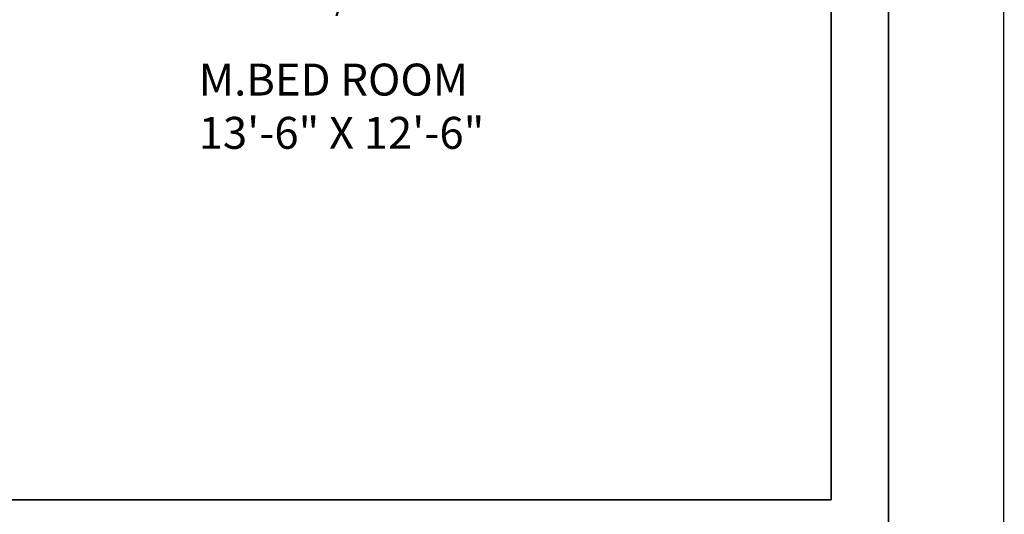
# Model space of a CAD drawing. Units: inches. Extents: x -638 to 186, y -762 to 59.
# Tile 22 of 31: x -125 to 29, y -203 to -126. Entities that reach past the tile are written whole.
import ezdxf

# ---------------------------------------------------------------- set-up
doc = ezdxf.new("R2010")
doc.units = ezdxf.units.IN
for name, color, linetype, lineweight in [('A-ANNO-DIMS', 2, 'Continuous', 18), ('A-AREA-IDEN', 1, 'Continuous', 18), ('C-PROP', 7, 'Continuous', 25), ('wall', 7, 'Continuous', 35)]:
    doc.layers.add(name, color=color, linetype=linetype, lineweight=lineweight)
doc.styles.get("Standard").update_dxf_attribs({"font": 'arial.ttf'})
doc.dimstyles.new('ISO-25', dxfattribs={"dimtxt": 4, "dimasz": 4, "dimexe": 1.25, "dimexo": 0.625, "dimtad": 0, "dimlunit": 4, "dimtxsty": 'Standard', "dimcen": 2.5, "dimclrt": 256, "dimadec": 0, "dimazin": 0, "dimtfac": 1, "dimtmove": 0, "dimatfit": 3, "dimfxl": 1, "dimfxlon": 1, "dimarcsym": 0})

# ---------------------------------------------------------------- blocks, each defined once
blk = doc.blocks.new('*D14')
at = {"layer": 'A-ANNO-DIMS', "color": 0, "lineweight": -2, "transparency": 16777216}
for p, q in [((45.41, -42.03), (47.66, -42.03)), ((46.41, -52.03), (46.41, -307.65)), ((46.41, -607.03), (46.41, -351.42)), ((45.41, -617.03), (47.66, -617.03))]:
    blk.add_line(p, q, dxfattribs=at)
at = {"layer": 'A-ANNO-DIMS', "color": 0, "lineweight": 30, "transparency": 16777216}
for points in [[(44.74, -52.03), (48.08, -52.03), (46.41, -42.03)], [(44.74, -607.03), (48.08, -607.03), (46.41, -617.03)]]:
    blk.add_solid(points, dxfattribs=at)
at = {"layer": 'Defpoints', "color": 0, "lineweight": 30, "transparency": 16777216}
for p in [(10.47, -42.03), (10.47, -617.03), (46.41, -617.03)]:
    blk.add_point(p, dxfattribs=at)
at = {"layer": 'A-ANNO-DIMS', "color": 0, "transparency": 16777216, "insert": (46.41, -329.53), "char_height": 10, "attachment_point": 5, "rotation": 90}
blk.add_mtext('47\'-11"', dxfattribs=at)
blk = doc.blocks.new('*D15')
at = {"layer": 'A-ANNO-DIMS', "color": 0, "lineweight": -2, "transparency": 16777216}
for p, q in [((69.33, -24.03), (71.58, -24.03)), ((70.33, -34.03), (70.33, -350.73)), ((70.33, -703.03), (70.33, -386.33)), ((69.33, -713.03), (71.58, -713.03))]:
    blk.add_line(p, q, dxfattribs=at)
at = {"layer": 'A-ANNO-DIMS', "color": 0, "lineweight": 30, "transparency": 16777216}
for points in [[(68.66, -34.03), (72, -34.03), (70.33, -24.03)], [(68.66, -703.03), (72, -703.03), (70.33, -713.03)]]:
    blk.add_solid(points, dxfattribs=at)
at = {"layer": 'Defpoints', "color": 0, "lineweight": 30, "transparency": 16777216}
for p in [(-24.67, -24.03), (-10.56, -713.03), (70.33, -713.03)]:
    blk.add_point(p, dxfattribs=at)
at = {"layer": 'A-ANNO-DIMS', "color": 0, "transparency": 16777216, "insert": (70.33, -368.53), "char_height": 10, "attachment_point": 5, "rotation": 90}
blk.add_mtext('57\'-5"', dxfattribs=at)
blk = doc.blocks.new('*D27')
at = {"layer": 'A-ANNO-DIMS', "color": 0, "lineweight": -2, "transparency": 16777216}
for p, q in [((-123.62, -121.82), (-123.62, -124.07)), ((-119.62, -122.82), (-114.39, -122.82)), ((-48.93, -122.82), (-54.16, -122.82)), ((-44.93, -121.82), (-44.93, -124.07))]:
    blk.add_line(p, q, dxfattribs=at)
at = {"layer": 'A-ANNO-DIMS', "color": 0, "lineweight": 30, "transparency": 16777216}
for points in [[(-119.62, -122.15), (-119.62, -123.48), (-123.62, -122.82)], [(-48.93, -122.15), (-48.93, -123.48), (-44.93, -122.82)]]:
    blk.add_solid(points, dxfattribs=at)
at = {"layer": 'Defpoints', "color": 0, "lineweight": 30, "transparency": 16777216}
for p in [(-123.62, -111.01), (-44.93, -111.01), (-44.93, -122.82)]:
    blk.add_point(p, dxfattribs=at)
at = {"layer": 'A-ANNO-DIMS', "transparency": 16777216, "insert": (-84.28, -122.82), "char_height": 4, "attachment_point": 5}
blk.add_mtext('BED SET 6\'-6 1/2" TYP.', dxfattribs=at)
blk = doc.blocks.new('*D49')
at = {"layer": 'A-ANNO-DIMS', "color": 0, "lineweight": -2, "transparency": 16777216}
for p, q in [((182.66, -144.8), (184.91, -144.8)), ((183.66, -148.8), (183.66, -154.33)), ((183.66, -171.81), (183.66, -166.28)), ((182.66, -175.81), (184.91, -175.81))]:
    blk.add_line(p, q, dxfattribs=at)
at = {"layer": 'A-ANNO-DIMS', "color": 0, "lineweight": 30, "transparency": 16777216}
for points in [[(183, -148.8), (184.33, -148.8), (183.66, -144.8)], [(183, -171.81), (184.33, -171.81), (183.66, -175.81)]]:
    blk.add_solid(points, dxfattribs=at)
at = {"layer": 'Defpoints', "color": 0, "lineweight": 30, "transparency": 16777216}
for p in [(-242.35, -144.8), (-242.35, -175.81), (183.66, -175.81)]:
    blk.add_point(p, dxfattribs=at)
at = {"layer": 'A-ANNO-DIMS', "transparency": 16777216, "insert": (183.66, -160.31), "char_height": 4, "attachment_point": 5, "rotation": 90}
blk.add_mtext('2\'-7"', dxfattribs=at)
blk = doc.blocks.new('*D56')
at = {"layer": 'A-ANNO-DIMS', "color": 0, "lineweight": -2, "transparency": 16777216}
for p, q in [((-165.03, 52.02), (-165.03, 54.27)), ((-100.53, 52.02), (-100.53, 54.27)), ((-161.03, 53.02), (-143.38, 53.02)), ((-104.53, 53.02), (-122.17, 53.02))]:
    blk.add_line(p, q, dxfattribs=at)
at = {"layer": 'A-ANNO-DIMS', "color": 0, "lineweight": 30, "transparency": 16777216}
for points in [[(-161.03, 53.68), (-161.03, 52.35), (-165.03, 53.02)], [(-104.53, 53.68), (-104.53, 52.35), (-100.53, 53.02)]]:
    blk.add_solid(points, dxfattribs=at)
at = {"layer": 'Defpoints', "color": 0, "lineweight": 30, "transparency": 16777216}
for p in [(-100.53, 53.02), (-165.03, -408.03), (-100.53, -408.03)]:
    blk.add_point(p, dxfattribs=at)
at = {"layer": 'A-ANNO-DIMS', "transparency": 16777216, "insert": (-132.78, 53.02), "char_height": 4, "attachment_point": 5}
blk.add_mtext('5\'-4 1/2"', dxfattribs=at)

msp = doc.modelspace()

# ---------------------------------------------------------------- linework, layer by layer
at = {"layer": 'C-PROP'}
msp.add_line((28.474, -24.033), (28.474, -713.033), dxfattribs=at)
at = {"layer": 'wall'}
for p, q in [((10.474, -42.033), (10.474, -617.033)), ((1.474, -51.033), (1.474, -201.033)), ((-160.526, -201.033), (1.474, -201.033))]:
    msp.add_line(p, q, dxfattribs=at)

# ---------------------------------------------------------------- texts
at = {"layer": 'A-AREA-IDEN', "insert": (-97.422, -132.728), "char_height": 5, "attachment_point": 1}
msp.add_mtext_dynamic_manual_height_columns('{M.BED ROOM\\P13\'-6" X 12\'-6"}', width=101.0374, gutter_width=12.5, heights=[0], dxfattribs=at)

# ---------------------------------------------------------------- dimensions: what is measured, and where the dimension line sits
at = {"layer": 'A-ANNO-DIMS'}
dim = msp.add_linear_dim(base=(-100.526, 53.017), p1=(-165.026, -408.033), p2=(-100.526, -408.033), dimstyle='ISO-25', override={"dimdec": 1, "dimlfac": 1, "dimrnd": 0, "dimzin": 1, "dimdsep": 46, "dimlunit": 4, "dimfrac": 2}, dxfattribs=at)
dim.commit()
dim.dimension.update_dxf_attribs({"geometry": '*D56', "text_midpoint": (-132.776, 53.017)})
for base, p1, p2, override, picture, middle in [((70.331, -713.033), (-24.669, -24.033), (-10.563, -713.033), {"dimtxt": 10, "dimasz": 10, "dimclrd": 0, "dimclre": 0, "dimclrt": 0}, '*D15', (70.331, -368.533)), ((46.411, -617.033), (10.474, -42.033), (10.474, -617.033), {"dimtxt": 10, "dimasz": 10, "dimclrd": 0, "dimclre": 0, "dimclrt": 0}, '*D14', (46.411, -329.533)), ((183.663, -175.813), (-242.352, -144.803), (-242.352, -175.813), {"dimdec": 1, "dimlfac": 1, "dimrnd": 0, "dimzin": 1, "dimdsep": 46, "dimlunit": 4, "dimfrac": 2}, '*D49', (183.663, -160.308))]:
    dim = msp.add_linear_dim(base=base, p1=p1, p2=p2, angle=90, dimstyle='ISO-25', override=override, dxfattribs=at)
    dim.commit()
    dim.dimension.update_dxf_attribs({"geometry": picture, "text_midpoint": middle})
dim = msp.add_linear_dim(base=(-44.925, -122.818), p1=(-123.625, -111.013), p2=(-44.925, -111.013), text='BED SET <> TYP.', dimstyle='ISO-25', override={"dimdec": 1, "dimlfac": 1, "dimrnd": 0, "dimzin": 1, "dimdsep": 46, "dimlunit": 4, "dimfrac": 2}, dxfattribs=at)
dim.commit()
dim.dimension.update_dxf_attribs({"geometry": '*D27', "text_midpoint": (-84.275, -122.818)})

doc.saveas('drawing.dxf')
